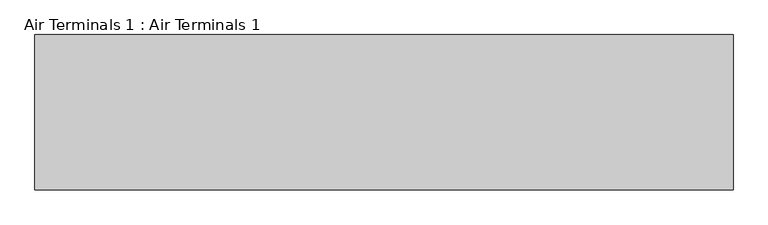
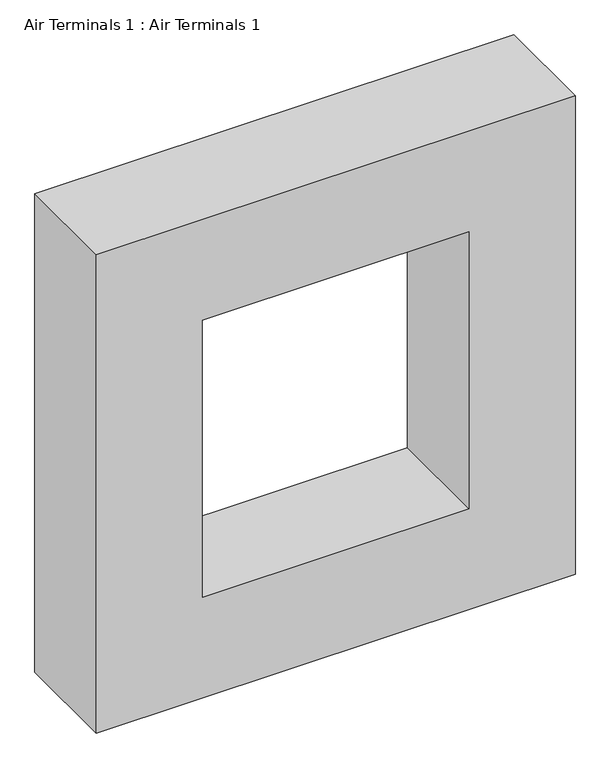
"""IFC4 building model written with IfcOpenShell, lengths in millimetres: air terminal geometry, Air Terminals 1 : Air Terminals 1."""

from ifc_helpers import new_model, si_unit, frame, origin, place, context, project, spatial, polyline, outline, extrude, source, transform, mapped, element, save


def air_terminals_1_air_terminals_1_01c5ecaf(model_context):
    return source(origin(), model_context, "Body", "SweptSolid", [
        extrude(outline(polyline([(7620.3519237, -13614.7873371), (7620.3519237, -14986.3873371), (6172.5519237, -14986.3873371), (6172.5519237, -13614.7873371), (7620.3519237, -13614.7873371)]), holes=[polyline([(7315.5519237, -13919.5873371), (6477.3519237, -13919.5873371), (6477.3519237, -14681.5873371), (7315.5519237, -14681.5873371), (7315.5519237, -13919.5873371)])]), frame((0.0, 3179.7527962, 0.0), z_axis=(0.0, 1.0, 0.0), x_axis=(0.0, 0.0, 1.0)), (0.0, 0.0, 1.0), 304.8),
    ])


if __name__ == "__main__":
    model = new_model("IFC4")
    model_context = context("Model", 3, world=origin())
    ifc_project = project(units=[si_unit("LENGTHUNIT", "METRE", prefix="MILLI")], contexts=[model_context])
    site = spatial("IfcSite", under=ifc_project)
    building = spatial("IfcBuilding", under=site)
    placement = place(None, origin())
    air_terminals_1_air_terminals_1_shape = air_terminals_1_air_terminals_1_01c5ecaf(model_context)
    element("IfcAirTerminal", 1, ObjectType="Air Terminals 1 : Air Terminals 1", at=placement, inside=building, context=model_context, shape_type="MappedRepresentation", body=[
        mapped(air_terminals_1_air_terminals_1_shape, transform((0.0, 0.0, 0.0), x_axis=(1.0, 0.0, 0.0), y_axis=(0.0, 1.0, 0.0), z_axis=(0.0, 0.0, 1.0))),
    ])
    save(model, "model.ifc")
